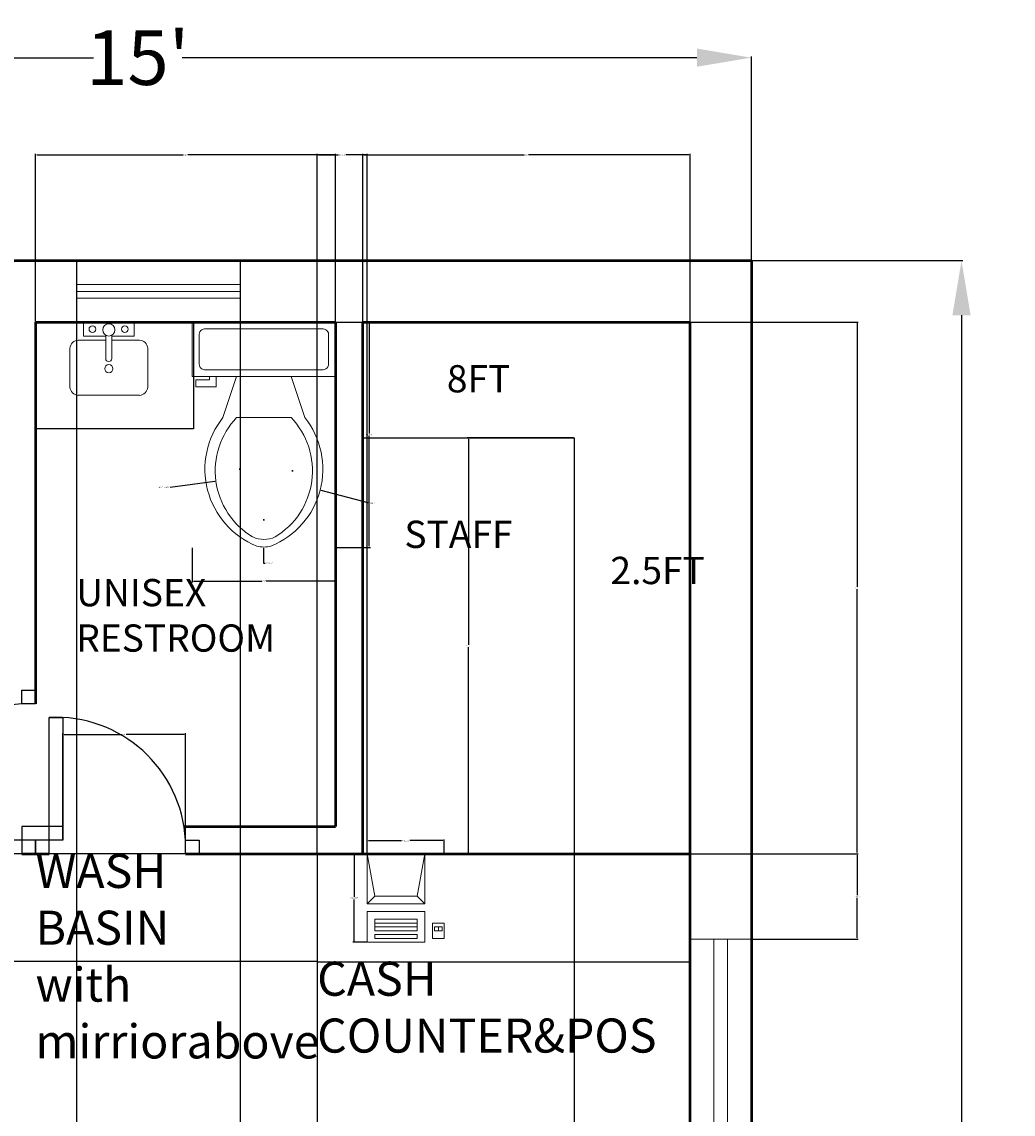
# Model space of a CAD drawing. Units: inches. Extents: x 226 to 1155, y 22 to 494.
# Tile 3 of 7: x 315 to 460, y 176 to 337. Entities that reach past the tile are written whole.
import ezdxf

# ---------------------------------------------------------------- set-up
doc = ezdxf.new("R2010")
doc.units = ezdxf.units.IN
doc.header["$MEASUREMENT"] = 0
for name, color, linetype, lineweight in [('A-ANNO-DIMS', 2, 'Continuous', 18), ('A-ANNO-TEXT', 7, 'Continuous', 18), ('A-AREA-IDEN', 7, 'Continuous', 25), ('A-DOOR', 3, 'Continuous', 25), ('A-EQPM', 8, 'Continuous', 18), ('A-FLOR-CASE', 9, 'Continuous', 25), ('A-FLOR-FIXT', 9, 'Continuous', 18), ('A-GLAZ', 4, 'Continuous', 18), ('A-WALL', 7, 'Continuous', 50)]:
    doc.layers.add(name, color=color, linetype=linetype, lineweight=lineweight)
doc.styles.get("Standard").update_dxf_attribs({"font": 'arial.ttf'})
doc.dimstyles.get("Standard").update_dxf_attribs({"dimtxt": 0.18, "dimasz": 0.18, "dimexe": 0.18, "dimexo": 0.0625, "dimgap": 0.09, "dimtad": 0, "dimtih": 1, "dimtoh": 1, "dimdec": 4, "dimzin": 0, "dimdsep": 46, "dimlunit": 4, "dimtxsty": 'Standard', "dimcen": 0.09, "dimadec": 0, "dimazin": 0, "dimtfac": 1, "dimtdec": 4, "dimtofl": 0, "dimtmove": 0, "dimatfit": 3, "dimfxl": 1, "dimtolj": 1, "dimtzin": 0, "dimarcsym": 0})

# ---------------------------------------------------------------- blocks, each defined once
blk = doc.blocks.new('Computer Terminal')
for p, q in [((-10, 11.5), (5, 11.5)), ((-8, 0.5), (-10, 11.5)), ((-10, -1.5), (-10, 11.5)), ((5, 11.5), (3, 0.5)), ((5, 11.5), (5, -1.5)), ((-10, -1.5), (-8, 0.5)), ((3, 0.5), (-8, 0.5)), ((3, 0.5), (5, -1.5)), ((5, -1.5), (-10, -1.5)), ((-10, -11.5), (-10, -3.5)), ((-10, -3.5), (5, -3.5)), ((-8, -5.5), (-8, -8.5)), ((3, -5.5), (-8, -5.5)), ((3, -8.5), (3, -5.5)), ((5, -3.5), (5, -11.5)), ((3, -6.5), (-8, -6.5)), ((-8, -7.5), (3, -7.5)), ((-8, -8.5), (3, -8.5)), ((10, -6.5), (7, -6.5)), ((7, -6.5), (7, -10.5)), ((9.5, -7.5), (7.5, -7.5)), ((7.5, -7.5), (7.5, -8.5)), ((7.5, -8.5), (9.5, -8.5)), ((8.5, -7.5), (8.5, -8.5)), ((9.5, -8.5), (9.5, -7.5)), ((10, -10.5), (10, -6.5)), ((-8, -9.5), (-8, -10.5)), ((3, -9.5), (-8, -9.5)), ((-8, -10.5), (3, -10.5)), ((3, -10.5), (3, -9.5)), ((7, -10.5), (10, -10.5)), ((5, -11.5), (-10, -11.5))]:
    blk.add_line(p, q)
blk = doc.blocks.new('Toilet - top')
for p, q in [((9.5, -6), (9.5, -2)), ((-8, -8.5), (-8, -8)), ((-7, -8), (-7, -9.5)), ((-4, -8), (-6, -14)), ((4, -8), (6, -14)), ((-10, -8.5), (-8, -8.5)), ((-10, -9.5), (-10, -8.5)), ((-7, -9.5), (-10, -9.5)), ((4, -14), (-4, -14))]:
    blk.add_line(p, q)
blk.add_lwpolyline([(10.5, -8), (10.5, 0), (-10.5, 0), (-10.5, -8)], close=True)
for points in [[(8.5, -1), (-8.5, -1)], [(-9.5, -2), (-9.5, -6)], [(-8.5, -7), (8.5, -7)]]:
    blk.add_lwpolyline(points)
for centre, radius, start, end in [((-8.62, -1.88), 0.884, 81.8699, 188.1301), ((8.62, -1.88), 0.884, 351.8699, 98.1301), ((-8.62, -6.12), 0.884, 171.8699, 278.1301), ((8.62, -6.12), 0.884, 261.8699, 8.1301), ((3.52, -21.58), 12.17, 141.4691, 247.9714), ((4.2, -21.82), 11.33, 136.3677, 238.9468), ((-3.52, -21.58), 12.17, 292.0284, 38.5307), ((-4.2, -21.82), 11.33, 301.053, 43.6321), ((0, -27.88), 4, 245.7318, 294.2682), ((0, -29), 4, 254.8605, 285.1395)]:
    blk.add_arc(centre, radius, start, end)
blk = doc.blocks.new('*D8')
at = {"layer": 'A-ANNO-DIMS', "color": 0, "lineweight": -2, "transparency": 16777216}
for p, q in [((421.77, 301.63), (452.71, 301.63)), ((452.53, 293.63), (452.53, 173.74)), ((452.53, 45.63), (452.53, 165.52)), ((421.77, 37.63), (452.71, 37.63))]:
    blk.add_line(p, q, dxfattribs=at)
at = {"layer": 'A-ANNO-DIMS', "color": 0, "transparency": 16777216}
for points in [[(451.2, 293.63), (453.86, 293.63), (452.53, 301.63)], [(451.2, 45.63), (453.86, 45.63), (452.53, 37.63)]]:
    blk.add_solid(points, dxfattribs=at)
at = {"layer": 'Defpoints', "color": 0, "transparency": 16777216}
for p in [(421.71, 301.63), (421.71, 37.63), (452.53, 37.63)]:
    blk.add_point(p, dxfattribs=at)
at = {"layer": 'A-ANNO-DIMS', "color": 0, "transparency": 16777216, "insert": (452.53, 169.63), "char_height": 8, "attachment_point": 5}
blk.add_mtext("\\A1;22'", dxfattribs=at)
blk = doc.blocks.new('*D9')
at = {"layer": 'A-ANNO-DIMS', "color": 0, "lineweight": -2, "transparency": 16777216}
for p, q in [((241.71, 301.69), (241.71, 331.58)), ((249.71, 331.4), (325.2, 331.4)), ((413.71, 331.4), (338.21, 331.4)), ((421.71, 301.69), (421.71, 331.58))]:
    blk.add_line(p, q, dxfattribs=at)
at = {"layer": 'A-ANNO-DIMS', "color": 0, "transparency": 16777216}
for points in [[(249.71, 332.74), (249.71, 330.07), (241.71, 331.4)], [(413.71, 332.74), (413.71, 330.07), (421.71, 331.4)]]:
    blk.add_solid(points, dxfattribs=at)
at = {"layer": 'Defpoints', "color": 0, "transparency": 16777216}
for p in [(421.71, 331.4), (241.71, 301.63), (421.71, 301.63)]:
    blk.add_point(p, dxfattribs=at)
at = {"layer": 'A-ANNO-DIMS', "color": 0, "transparency": 16777216, "insert": (331.71, 331.4), "char_height": 8, "attachment_point": 5}
blk.add_mtext("\\A1;15'", dxfattribs=at)
blk = doc.blocks.new('BASIN-WITH-FAUCET')
blk.add_line((6.15, 5.4), (6.15, 8.82))
for points in [[(5.25, 8.7), (2, 8.7), (2, 10.75), (5.8, 10.75)], [(5.8, 10.75), (9.4, 10.75), (9.4, 8.7), (6.15, 8.7)], [(1.2, 8.1), (5.25, 8.1)], [(6.15, 8.1), (10.2, 8.1)], [(0, 1.2), (0, 6.9)], [(11.4, 6.9), (11.4, 1.2)], [(10.2, 0), (1.2, 0)]]:
    blk.add_lwpolyline(points)
blk.add_lwpolyline([(6.15, 5.4, -1), (5.25, 5.4), (5.25, 8.82)], format="xyb")
for centre, radius in [((3.3, 9.7), 0.5), ((5.7, 9.6), 0.9), ((8.05, 9.7), 0.5), ((5.7, 3.9), 0.6)]:
    blk.add_circle(centre, radius)
for centre, start, end in [((1.28, 6.82), 93.3665, 176.6335), ((10.13, 6.82), 3.3665, 86.6335), ((1.28, 1.27), 183.3665, 266.6335), ((10.13, 1.27), 273.3665, 356.6335)]:
    blk.add_arc(centre, 1.28, start, end)
blk = doc.blocks.new('WIN-36')
for p, q in [((0, 5.5), (36, 5.5)), ((0, 3.5), (36, 3.5))]:
    blk.add_line(p, q)
blk.add_lwpolyline([(36, 9), (36, 0), (0, 0), (0, 9)], close=True)
blk = doc.blocks.new('*D46')
at = {"layer": 'A-ANNO-DIMS', "color": 0, "lineweight": -2, "transparency": 16777216}
for p, q in [((365.31, 214.63), (363.25, 214.63)), ((363.43, 214.45), (363.43, 208.33)), ((363.43, 201.84), (363.43, 207.96)), ((365.31, 201.66), (363.25, 201.66))]:
    blk.add_line(p, q, dxfattribs=at)
at = {"layer": 'A-ANNO-DIMS', "color": 0, "transparency": 16777216}
for points in [[(363.4, 214.45), (363.46, 214.45), (363.43, 214.63)], [(363.4, 201.84), (363.46, 201.84), (363.43, 201.66)]]:
    blk.add_solid(points, dxfattribs=at)
at = {"layer": 'Defpoints', "color": 0, "transparency": 16777216}
for p in [(363.43, 214.63), (365.38, 214.63), (365.38, 201.66)]:
    blk.add_point(p, dxfattribs=at)
at = {"layer": 'A-ANNO-DIMS', "color": 0, "transparency": 16777216, "insert": (363.43, 208.15), "char_height": 0.18, "attachment_point": 5}
blk.add_mtext('\\A1;POS 1\'-1"', dxfattribs=at)
blk = doc.blocks.new('*D47')
at = {"layer": 'A-ANNO-DIMS', "color": 0, "lineweight": -2, "transparency": 16777216}
for p, q in [((365.38, 214.69), (365.38, 216.76)), ((365.56, 216.58), (370.41, 216.58)), ((376.47, 216.58), (371.62, 216.58)), ((376.65, 214.69), (376.65, 216.76))]:
    blk.add_line(p, q, dxfattribs=at)
at = {"layer": 'A-ANNO-DIMS', "color": 0, "transparency": 16777216}
for points in [[(365.56, 216.61), (365.56, 216.55), (365.38, 216.58)], [(376.47, 216.61), (376.47, 216.55), (376.65, 216.58)]]:
    blk.add_solid(points, dxfattribs=at)
at = {"layer": 'Defpoints', "color": 0, "transparency": 16777216}
for p in [(376.65, 216.58), (365.38, 214.63), (376.65, 214.63)]:
    blk.add_point(p, dxfattribs=at)
at = {"layer": 'A-ANNO-DIMS', "color": 0, "transparency": 16777216, "insert": (371.01, 216.58), "char_height": 0.18, "attachment_point": 5}
blk.add_mtext('\\A1;0\'-11 1/2"', dxfattribs=at)
blk = doc.blocks.new('*D54')
at = {"layer": 'A-ANNO-DIMS', "color": 0, "lineweight": -2, "transparency": 16777216}
for p, q in [((360.77, 292.63), (365.84, 292.63)), ((365.66, 292.45), (365.66, 276.29)), ((365.66, 259.76), (365.66, 275.92)), ((360.77, 259.58), (365.84, 259.58))]:
    blk.add_line(p, q, dxfattribs=at)
at = {"layer": 'A-ANNO-DIMS', "color": 0, "transparency": 16777216}
for points in [[(365.63, 292.45), (365.69, 292.45), (365.66, 292.63)], [(365.63, 259.76), (365.69, 259.76), (365.66, 259.58)]]:
    blk.add_solid(points, dxfattribs=at)
at = {"layer": 'Defpoints', "color": 0, "transparency": 16777216}
for p in [(360.71, 292.63), (365.66, 292.63), (360.71, 259.58)]:
    blk.add_point(p, dxfattribs=at)
at = {"layer": 'A-ANNO-DIMS', "color": 0, "transparency": 16777216, "insert": (365.66, 276.11), "char_height": 0.18, "attachment_point": 5}
blk.add_mtext('\\A1;WC 2\'-9"', dxfattribs=at)
blk = doc.blocks.new('*D55')
at = {"layer": 'A-ANNO-DIMS', "color": 0, "lineweight": -2, "transparency": 16777216}
for p, q in [((339.71, 259.52), (339.71, 254.45)), ((360.71, 259.52), (360.71, 254.45)), ((339.89, 254.63), (349.89, 254.63)), ((360.53, 254.63), (350.53, 254.63))]:
    blk.add_line(p, q, dxfattribs=at)
at = {"layer": 'A-ANNO-DIMS', "color": 0, "transparency": 16777216}
for points in [[(339.89, 254.66), (339.89, 254.6), (339.71, 254.63)], [(360.53, 254.66), (360.53, 254.6), (360.71, 254.63)]]:
    blk.add_solid(points, dxfattribs=at)
at = {"layer": 'Defpoints', "color": 0, "transparency": 16777216}
for p in [(339.71, 259.58), (360.71, 259.58), (360.71, 254.63)]:
    blk.add_point(p, dxfattribs=at)
at = {"layer": 'A-ANNO-DIMS', "color": 0, "transparency": 16777216, "insert": (350.21, 254.63), "char_height": 0.18, "attachment_point": 5}
blk.add_mtext('\\A1;1\'-9"', dxfattribs=at)
blk = doc.blocks.new('*D57')
at = {"layer": 'A-ANNO-DIMS', "color": 0, "lineweight": -2, "transparency": 16777216}
for p, q in [((316.71, 292.69), (316.71, 317.31)), ((360.71, 292.69), (360.71, 317.31)), ((316.89, 317.13), (338.38, 317.13)), ((360.53, 317.13), (339.04, 317.13))]:
    blk.add_line(p, q, dxfattribs=at)
at = {"layer": 'A-ANNO-DIMS', "color": 0, "transparency": 16777216}
for points in [[(316.89, 317.16), (316.89, 317.1), (316.71, 317.13)], [(360.53, 317.16), (360.53, 317.1), (360.71, 317.13)]]:
    blk.add_solid(points, dxfattribs=at)
at = {"layer": 'Defpoints', "color": 0, "transparency": 16777216}
for p in [(360.71, 317.13), (316.71, 292.63), (360.71, 292.63)]:
    blk.add_point(p, dxfattribs=at)
at = {"layer": 'A-ANNO-DIMS', "color": 0, "transparency": 16777216, "insert": (338.71, 317.13), "char_height": 0.18, "attachment_point": 5}
blk.add_mtext('\\A1;3\'-8"', dxfattribs=at)
blk = doc.blocks.new('*D58')
at = {"layer": 'A-ANNO-DIMS', "color": 0, "lineweight": -2, "transparency": 16777216}
for p, q in [((364.71, 292.69), (364.71, 317.31)), ((412.71, 292.69), (412.71, 317.31)), ((364.89, 317.13), (388.37, 317.13)), ((412.53, 317.13), (389.04, 317.13))]:
    blk.add_line(p, q, dxfattribs=at)
at = {"layer": 'A-ANNO-DIMS', "color": 0, "transparency": 16777216}
for points in [[(364.89, 317.16), (364.89, 317.1), (364.71, 317.13)], [(412.53, 317.16), (412.53, 317.1), (412.71, 317.13)]]:
    blk.add_solid(points, dxfattribs=at)
at = {"layer": 'Defpoints', "color": 0, "transparency": 16777216}
for p in [(412.71, 317.13), (364.71, 292.63), (412.71, 292.63)]:
    blk.add_point(p, dxfattribs=at)
at = {"layer": 'A-ANNO-DIMS', "color": 0, "transparency": 16777216, "insert": (388.71, 317.13), "char_height": 0.18, "attachment_point": 5}
blk.add_mtext('\\A1;4\'-0"', dxfattribs=at)
blk = doc.blocks.new('*D60')
at = {"layer": 'A-ANNO-DIMS', "color": 0, "lineweight": -2, "transparency": 16777216}
for p, q in [((412.77, 292.63), (437.39, 292.63)), ((437.21, 292.45), (437.21, 253.81)), ((437.21, 214.81), (437.21, 253.45)), ((412.77, 214.63), (437.39, 214.63))]:
    blk.add_line(p, q, dxfattribs=at)
at = {"layer": 'A-ANNO-DIMS', "color": 0, "transparency": 16777216}
for points in [[(437.18, 292.45), (437.24, 292.45), (437.21, 292.63)], [(437.18, 214.81), (437.24, 214.81), (437.21, 214.63)]]:
    blk.add_solid(points, dxfattribs=at)
at = {"layer": 'Defpoints', "color": 0, "transparency": 16777216}
for p in [(412.71, 292.63), (437.21, 292.63), (412.71, 214.63)]:
    blk.add_point(p, dxfattribs=at)
at = {"layer": 'A-ANNO-DIMS', "color": 0, "transparency": 16777216, "insert": (437.21, 253.63), "char_height": 0.18, "attachment_point": 5}
blk.add_mtext('\\A1;6\'-6"', dxfattribs=at)
blk = doc.blocks.new('*D66')
at = {"layer": 'A-ANNO-DIMS', "color": 0, "lineweight": -2, "transparency": 16777216}
for p, q in [((412.77, 214.63), (437.39, 214.63)), ((437.21, 214.45), (437.21, 208.56)), ((437.21, 202.29), (437.21, 208.19)), ((421.77, 202.11), (437.39, 202.11))]:
    blk.add_line(p, q, dxfattribs=at)
at = {"layer": 'A-ANNO-DIMS', "color": 0, "transparency": 16777216}
for points in [[(437.18, 214.45), (437.24, 214.45), (437.21, 214.63)], [(437.18, 202.29), (437.24, 202.29), (437.21, 202.11)]]:
    blk.add_solid(points, dxfattribs=at)
at = {"layer": 'Defpoints', "color": 0, "transparency": 16777216}
for p in [(412.71, 214.63), (437.21, 214.63), (421.71, 202.11)]:
    blk.add_point(p, dxfattribs=at)
at = {"layer": 'A-ANNO-DIMS', "color": 0, "transparency": 16777216, "insert": (437.21, 208.37), "char_height": 0.18, "attachment_point": 5}
blk.add_mtext('\\A1;1\'-0 1/2"', dxfattribs=at)
blk = doc.blocks.new('*D71')
at = {"layer": 'A-ANNO-DIMS', "color": 0, "lineweight": -2, "transparency": 16777216}
for p, q in [((241.71, 301.57), (241.71, 21.95)), ((322.71, 301.57), (322.71, 21.95)), ((241.89, 22.13), (281.88, 22.13)), ((322.53, 22.13), (282.54, 22.13))]:
    blk.add_line(p, q, dxfattribs=at)
at = {"layer": 'A-ANNO-DIMS', "color": 0, "transparency": 16777216}
for points in [[(241.89, 22.16), (241.89, 22.1), (241.71, 22.13)], [(322.53, 22.16), (322.53, 22.1), (322.71, 22.13)]]:
    blk.add_solid(points, dxfattribs=at)
at = {"layer": 'Defpoints', "color": 0, "transparency": 16777216}
for p in [(241.71, 301.63), (322.71, 301.63), (322.71, 22.13)]:
    blk.add_point(p, dxfattribs=at)
at = {"layer": 'A-ANNO-DIMS', "color": 0, "transparency": 16777216, "insert": (282.21, 22.13), "char_height": 0.18, "attachment_point": 5}
blk.add_mtext('\\A1;6\'-9"', dxfattribs=at)
blk = doc.blocks.new('*D72')
at = {"layer": 'A-ANNO-DIMS', "color": 0, "lineweight": -2, "transparency": 16777216}
for p, q in [((322.71, 301.57), (322.71, 21.95)), ((346.71, 301.57), (346.71, 21.95)), ((322.89, 22.13), (334.38, 22.13)), ((346.53, 22.13), (335.04, 22.13))]:
    blk.add_line(p, q, dxfattribs=at)
at = {"layer": 'A-ANNO-DIMS', "color": 0, "transparency": 16777216}
for points in [[(322.89, 22.16), (322.89, 22.1), (322.71, 22.13)], [(346.53, 22.16), (346.53, 22.1), (346.71, 22.13)]]:
    blk.add_solid(points, dxfattribs=at)
at = {"layer": 'Defpoints', "color": 0, "transparency": 16777216}
for p in [(322.71, 301.63), (346.71, 301.63), (346.71, 22.13)]:
    blk.add_point(p, dxfattribs=at)
at = {"layer": 'A-ANNO-DIMS', "color": 0, "transparency": 16777216, "insert": (334.71, 22.13), "char_height": 0.18, "attachment_point": 5}
blk.add_mtext('\\A1;2\'-0"', dxfattribs=at)
blk = doc.blocks.new('*D81')
at = {"layer": 'A-ANNO-DIMS', "color": 0, "lineweight": -2, "transparency": 16777216}
for p, q in [((358.02, 198.75), (358.02, 21.95)), ((412.71, 198.75), (412.71, 21.95)), ((358.2, 22.13), (384.82, 22.13)), ((412.53, 22.13), (385.91, 22.13))]:
    blk.add_line(p, q, dxfattribs=at)
at = {"layer": 'A-ANNO-DIMS', "color": 0, "transparency": 16777216}
for points in [[(358.2, 22.16), (358.2, 22.1), (358.02, 22.13)], [(412.53, 22.16), (412.53, 22.1), (412.71, 22.13)]]:
    blk.add_solid(points, dxfattribs=at)
at = {"layer": 'Defpoints', "color": 0, "transparency": 16777216}
for p in [(358.02, 198.82), (412.71, 198.82), (412.71, 22.13)]:
    blk.add_point(p, dxfattribs=at)
at = {"layer": 'A-ANNO-DIMS', "color": 0, "transparency": 16777216, "insert": (385.36, 22.13), "char_height": 0.18, "attachment_point": 5}
blk.add_mtext('\\A1;4\'-6 1/2"', dxfattribs=at)
blk = doc.blocks.new('*D82')
at = {"layer": 'A-ANNO-DIMS', "color": 0, "lineweight": -2, "transparency": 16777216}
for p, q in [((357.96, 214.63), (226.03, 214.63)), ((226.21, 214.45), (226.21, 206.9)), ((226.21, 199), (226.21, 206.54)), ((357.96, 198.82), (226.03, 198.82))]:
    blk.add_line(p, q, dxfattribs=at)
at = {"layer": 'A-ANNO-DIMS', "color": 0, "transparency": 16777216}
for points in [[(226.18, 214.45), (226.24, 214.45), (226.21, 214.63)], [(226.18, 199), (226.24, 199), (226.21, 198.82)]]:
    blk.add_solid(points, dxfattribs=at)
at = {"layer": 'Defpoints', "color": 0, "transparency": 16777216}
for p in [(226.21, 214.63), (358.02, 214.63), (358.02, 198.82)]:
    blk.add_point(p, dxfattribs=at)
at = {"layer": 'A-ANNO-DIMS', "color": 0, "transparency": 16777216, "insert": (226.21, 206.72), "char_height": 0.18, "attachment_point": 5}
blk.add_mtext('\\A1;1\'-4"', dxfattribs=at)
blk = doc.blocks.new('*D83')
at = {"layer": 'A-ANNO-DIMS', "color": 0, "lineweight": -2, "transparency": 16777216}
for p, q in [((358.02, 214.69), (358.02, 317.31)), ((365.38, 214.69), (365.38, 317.31)), ((358.2, 317.13), (361.16, 317.13)), ((365.2, 317.13), (362.24, 317.13))]:
    blk.add_line(p, q, dxfattribs=at)
at = {"layer": 'A-ANNO-DIMS', "color": 0, "transparency": 16777216}
for points in [[(358.2, 317.16), (358.2, 317.1), (358.02, 317.13)], [(365.2, 317.16), (365.2, 317.1), (365.38, 317.13)]]:
    blk.add_solid(points, dxfattribs=at)
at = {"layer": 'Defpoints', "color": 0, "transparency": 16777216}
for p in [(365.38, 317.13), (358.02, 214.63), (365.38, 214.63)]:
    blk.add_point(p, dxfattribs=at)
at = {"layer": 'A-ANNO-DIMS', "color": 0, "transparency": 16777216, "insert": (361.7, 317.13), "char_height": 0.18, "attachment_point": 5}
blk.add_mtext('\\A1;0\'-7 1/2"', dxfattribs=at)
blk = doc.blocks.new('*D84')
at = {"layer": 'A-ANNO-DIMS', "color": 0, "lineweight": -2, "transparency": 16777216}
for p, q in [((412.71, 292.57), (412.71, 21.95)), ((395.71, 275.57), (395.71, 21.95)), ((395.89, 22.13), (403.89, 22.13)), ((412.53, 22.13), (404.53, 22.13))]:
    blk.add_line(p, q, dxfattribs=at)
at = {"layer": 'A-ANNO-DIMS', "color": 0, "transparency": 16777216}
for points in [[(395.89, 22.16), (395.89, 22.1), (395.71, 22.13)], [(412.53, 22.16), (412.53, 22.1), (412.71, 22.13)]]:
    blk.add_solid(points, dxfattribs=at)
at = {"layer": 'Defpoints', "color": 0, "transparency": 16777216}
for p in [(412.71, 292.63), (395.71, 275.63), (412.71, 22.13)]:
    blk.add_point(p, dxfattribs=at)
at = {"layer": 'A-ANNO-DIMS', "color": 0, "transparency": 16777216, "insert": (404.21, 22.13), "char_height": 0.18, "attachment_point": 5}
blk.add_mtext('\\A1;1\'-5"', dxfattribs=at)
blk = doc.blocks.new('*D85')
at = {"layer": 'A-ANNO-DIMS', "color": 0, "lineweight": -2, "transparency": 16777216}
for p, q in [((395.64, 275.63), (380.03, 275.63)), ((380.21, 275.45), (380.21, 245.31)), ((380.21, 214.81), (380.21, 244.95)), ((395.64, 214.63), (380.03, 214.63))]:
    blk.add_line(p, q, dxfattribs=at)
at = {"layer": 'A-ANNO-DIMS', "color": 0, "transparency": 16777216}
for points in [[(380.18, 275.45), (380.24, 275.45), (380.21, 275.63)], [(380.18, 214.81), (380.24, 214.81), (380.21, 214.63)]]:
    blk.add_solid(points, dxfattribs=at)
at = {"layer": 'Defpoints', "color": 0, "transparency": 16777216}
for p in [(380.21, 275.63), (395.71, 275.63), (395.71, 214.63)]:
    blk.add_point(p, dxfattribs=at)
at = {"layer": 'A-ANNO-DIMS', "color": 0, "transparency": 16777216, "insert": (380.21, 245.13), "char_height": 0.18, "attachment_point": 5}
blk.add_mtext('\\A1;5\'-1"', dxfattribs=at)
blk = doc.blocks.new('*D90')
at = {"layer": 'A-ANNO-DIMS', "color": 0, "lineweight": -2, "transparency": 16777216}
for p, q in [((320.71, 216.69), (320.71, 232.31)), ((338.71, 216.69), (338.71, 232.31)), ((320.89, 232.13), (329.39, 232.13)), ((338.53, 232.13), (330.03, 232.13))]:
    blk.add_line(p, q, dxfattribs=at)
at = {"layer": 'A-ANNO-DIMS', "color": 0, "transparency": 16777216}
for points in [[(320.89, 232.16), (320.89, 232.1), (320.71, 232.13)], [(338.53, 232.16), (338.53, 232.1), (338.71, 232.13)]]:
    blk.add_solid(points, dxfattribs=at)
at = {"layer": 'Defpoints', "color": 0, "transparency": 16777216}
for p in [(338.71, 232.13), (320.71, 216.63), (338.71, 216.63)]:
    blk.add_point(p, dxfattribs=at)
at = {"layer": 'A-ANNO-DIMS', "color": 0, "transparency": 16777216, "insert": (329.71, 232.13), "char_height": 0.18, "attachment_point": 5}
blk.add_mtext('\\A1;1\'-6"', dxfattribs=at)
blk = doc.blocks.new('*D120')
at = {"layer": 'A-ANNO-DIMS', "color": 0, "lineweight": -2, "transparency": 16777216}
for p, q in [((346.6, 271.05), (346.78, 271.05)), ((346.69, 270.96), (346.69, 271.14)), ((365.52, 266.1), (358.63, 267.91))]:
    blk.add_line(p, q, dxfattribs=at)
at = {"layer": 'A-ANNO-DIMS', "color": 0, "transparency": 16777216}
blk.add_solid([(358.64, 267.94), (358.62, 267.88), (358.46, 267.96)], dxfattribs=at)
at = {"layer": 'Defpoints', "color": 0, "transparency": 16777216}
for p in [(346.69, 271.05), (358.46, 267.96)]:
    blk.add_point(p, dxfattribs=at)
at = {"layer": 'A-ANNO-DIMS', "color": 0, "transparency": 16777216, "insert": (366.13, 266.1), "char_height": 0.18, "attachment_point": 5}
blk.add_mtext('\\A1;2X R1\'-0"', dxfattribs=at)
blk = doc.blocks.new('*D121')
at = {"layer": 'A-ANNO-DIMS', "color": 0, "lineweight": -2, "transparency": 16777216}
for p, q in [((354.32, 270.81), (354.5, 270.81)), ((354.41, 270.72), (354.41, 270.9)), ((336.44, 268.4), (343, 269.28))]:
    blk.add_line(p, q, dxfattribs=at)
at = {"layer": 'A-ANNO-DIMS', "color": 0, "transparency": 16777216}
blk.add_solid([(343, 269.31), (343, 269.25), (343.18, 269.3)], dxfattribs=at)
at = {"layer": 'Defpoints', "color": 0, "transparency": 16777216}
for p in [(354.41, 270.81), (343.18, 269.3)]:
    blk.add_point(p, dxfattribs=at)
at = {"layer": 'A-ANNO-DIMS', "color": 0, "transparency": 16777216, "insert": (335.55, 268.4), "char_height": 0.18, "attachment_point": 5}
blk.add_mtext('\\A1;2X R0\'-11 1/2"', dxfattribs=at)
blk = doc.blocks.new('*D122')
at = {"layer": 'A-ANNO-DIMS', "color": 0, "lineweight": -2, "transparency": 16777216}
for p, q in [((350.12, 263.63), (350.3, 263.63)), ((350.21, 263.54), (350.21, 263.72)), ((350.21, 257.23), (350.21, 259.45)), ((350.39, 257.23), (350.21, 257.23))]:
    blk.add_line(p, q, dxfattribs=at)
at = {"layer": 'A-ANNO-DIMS', "color": 0, "transparency": 16777216}
blk.add_solid([(350.24, 259.45), (350.18, 259.45), (350.21, 259.63)], dxfattribs=at)
at = {"layer": 'Defpoints', "color": 0, "transparency": 16777216}
for p in [(350.21, 263.63), (350.21, 259.63)]:
    blk.add_point(p, dxfattribs=at)
at = {"layer": 'A-ANNO-DIMS', "color": 0, "transparency": 16777216, "insert": (351, 257.23), "char_height": 0.18, "attachment_point": 5}
blk.add_mtext('\\A1;2X R0\'-4"', dxfattribs=at)

msp = doc.modelspace()

# ---------------------------------------------------------------- linework, layer by layer
at = {"layer": 'A-DOOR'}
for p, q in [((316.70585, 236.62988), (316.70585, 238.62988)), ((316.70585, 214.62988), (316.70585, 216.62988)), ((316.70585, 214.62988), (318.70585, 214.62988)), ((338.70585, 214.62988), (340.70585, 214.62988))]:
    msp.add_line(p, q, dxfattribs=at)
for points in [[(316.70585, 238.62988), (316.70585, 236.62988), (314.70585, 236.62988), (314.70585, 238.62988)], [(316.70585, 214.62988), (316.70585, 216.62988), (314.70585, 216.62988), (314.70585, 214.62988)], [(316.70585, 214.62988), (318.70585, 214.62988), (318.70585, 216.62988), (316.70585, 216.62988)], [(340.70585, 214.62988), (338.70585, 214.62988), (338.70585, 216.62988), (340.70585, 216.62988)]]:
    msp.add_lwpolyline(points, close=True, dxfattribs=at)
for points in [[(314.70585, 236.62988, 0.414213562), (296.70585, 216.62988), (296.70585, 218.62988)], [(338.70585, 216.62988, 0.414213562), (318.70585, 234.62988), (320.70585, 234.62988), (320.70585, 216.62988), (318.70585, 216.62988), (318.70585, 234.62988)]]:
    msp.add_lwpolyline(points, format="xyb", dxfattribs=at)
msp.add_lwpolyline([(320.70585, 218.62988), (314.70585, 218.62988), (314.70585, 216.62988), (296.70585, 216.62988)], dxfattribs=at)
at = {"layer": 'A-EQPM'}
msp.add_line((365.37517, 214.62988), (373.83336, 214.62988), dxfattribs=at)
at = {"layer": 'A-FLOR-CASE'}
msp.add_lwpolyline([(316.70585, 292.62988), (339.86098, 292.62988), (339.86098, 276.95966), (316.70585, 276.95966)], close=True, dxfattribs=at)
for points in [[(364.70585, 275.62988), (395.70585, 275.62988), (395.70585, 214.62988)], [(358.02219, 214.62988), (358.02219, 198.81719), (412.70585, 198.81719)]]:
    msp.add_lwpolyline(points, dxfattribs=at)
at = {"layer": 'A-GLAZ'}
for p, q in [((322.7094, 298.12988), (346.7094, 298.12988)), ((322.7094, 297.12988), (346.7094, 297.12988)), ((322.7094, 296.12988), (346.7094, 296.12988))]:
    msp.add_line(p, q, dxfattribs=at)
msp.add_lwpolyline([(346.7094, 301.62988), (346.7094, 292.62988), (322.7094, 292.62988), (322.7094, 301.62988)], close=True, dxfattribs=at)
at = {"layer": 'A-WALL'}
for p, q in [((316.70585, 292.62988), (316.70585, 236.62988)), ((316.70585, 292.62988), (360.70585, 292.62988)), ((360.70585, 292.62988), (360.70585, 218.62988)), ((338.49414, 218.62988), (360.70585, 218.62988)), ((314.70585, 214.62988), (318.70585, 214.62988)), ((338.70585, 214.62988), (412.70585, 214.62988))]:
    msp.add_line(p, q, dxfattribs=at)
for points in [[(307.38052, 37.62988), (241.70585, 37.62988), (241.70585, 301.62988), (421.70585, 301.62988), (421.70585, 37.62988), (351.38052, 37.62988)], [(364.70585, 214.62988), (364.70585, 292.62988), (412.70585, 292.62988), (412.70585, 46.62988), (349.38052, 46.62988)]]:
    msp.add_lwpolyline(points, dxfattribs=at)

# ---------------------------------------------------------------- block references
at = {"layer": 'A-EQPM', "xscale": 0.56387934998791, "yscale": 0.56387934998791, "zscale": 0.56387934998791}
msp.add_blockref('Computer Terminal', (371.01397, 208.14526), dxfattribs=at)
at = {"layer": 'A-FLOR-FIXT'}
for name, p in [('BASIN-WITH-FAUCET', (321.761, 281.88)), ('Toilet - top', (350.20585, 292.62988))]:
    msp.add_blockref(name, p, dxfattribs=at)
at = {"layer": 'A-GLAZ', "rotation": 270}
msp.add_blockref('WIN-36', (412.70597, 202.11457), dxfattribs=at)

# ---------------------------------------------------------------- texts
at = {"layer": 'A-ANNO-TEXT', "attachment_point": 1}
for s, width, insert, char_height in [('8FT', 14.5329901, (377.0411, 286.3119), 4), ('2.5FT', 7.61252, (401.03207, 258.19169), 4), ('WASH BASIN\\Pwith mirriorabove', 32.3909522, (316.70585, 214.62988), 5), ('CASH COUNTER&POS', 54.6836594, (358.02219, 198.81719), 5)]:
    msp.add_mtext_dynamic_manual_height_columns(s, width=width, gutter_width=1, heights=[0], dxfattribs=dict(at, insert=insert, char_height=char_height))
at = {"layer": 'A-AREA-IDEN', "char_height": 4, "attachment_point": 1}
for s, width, insert in [('STAFF ', 21.2227815, (370.81267, 263.49304)), ('UNISEX\\PRESTROOM', 38.0282515, (322.67759, 254.94662))]:
    msp.add_mtext_dynamic_manual_height_columns(s, width=width, gutter_width=1, heights=[0], dxfattribs=dict(at, insert=insert))

# ---------------------------------------------------------------- dimensions: what is measured, and where the dimension line sits
at = {"layer": 'A-ANNO-DIMS'}
for base, p1, p2, override, picture, middle in [((421.70585, 331.40497), (241.70585, 301.62988), (421.70585, 301.62988), {"dimtxt": 8, "dimasz": 8, "dimclrd": 0, "dimclre": 0, "dimclrt": 0}, '*D9', (331.70585, 331.40497)), ((360.70585, 317.12988), (316.70585, 292.62988), (360.70585, 292.62988), {"dimdec": 1, "dimlfac": 1, "dimrnd": 0, "dimzin": 1, "dimdsep": 46, "dimlunit": 4, "dimfrac": 2}, '*D57', (338.70585, 317.12988)), ((365.37517, 317.12988), (358.02219, 214.62988), (365.37517, 214.62988), {"dimdec": 1, "dimlfac": 1, "dimrnd": 0, "dimzin": 1, "dimdsep": 46, "dimlunit": 4, "dimfrac": 2}, '*D83', (361.69868, 317.12988)), ((412.70584, 317.12988), (364.70585, 292.62988), (412.70584, 292.62988), {"dimdec": 1, "dimlfac": 1, "dimrnd": 0, "dimzin": 1, "dimdsep": 46, "dimlunit": 4, "dimfrac": 2}, '*D58', (388.70585, 317.12988)), ((322.7094, 22.12988), (241.70585, 301.62988), (322.7094, 301.62988), {"dimdec": 1, "dimlfac": 1, "dimrnd": 0, "dimzin": 1, "dimdsep": 46, "dimlunit": 4, "dimfrac": 2}, '*D71', (282.20762, 22.12988)), ((346.7094, 22.12988), (322.7094, 301.62988), (346.7094, 301.62988), {"dimdec": 1, "dimlfac": 1, "dimrnd": 0, "dimzin": 1, "dimdsep": 46, "dimlunit": 4, "dimfrac": 2}, '*D72', (334.7094, 22.12988)), ((412.70584, 22.12988), (395.70585, 275.62988), (412.70584, 292.62988), {"dimdec": 1, "dimlfac": 1, "dimrnd": 0, "dimzin": 1, "dimdsep": 46, "dimlunit": 4, "dimfrac": 2}, '*D84', (404.20584, 22.12988)), ((360.70585, 254.6267), (339.70585, 259.58363), (360.70585, 259.58363), {"dimdec": 1, "dimlfac": 1, "dimrnd": 0, "dimzin": 1, "dimdsep": 46, "dimlunit": 4, "dimfrac": 2}, '*D55', (350.20585, 254.6267)), ((338.70585, 232.12988), (320.70585, 216.62988), (338.70585, 216.62988), {"dimdec": 1, "dimlfac": 1, "dimrnd": 0, "dimzin": 1, "dimdsep": 46, "dimlunit": 4, "dimfrac": 2}, '*D90', (329.70585, 232.12988)), ((376.65276, 216.57526), (365.37517, 214.62988), (376.65276, 214.62988), {"dimdec": 1, "dimlfac": 1, "dimrnd": 0, "dimzin": 1, "dimdsep": 46, "dimlunit": 4, "dimfrac": 2}, '*D47', (371.01397, 216.57526)), ((412.70584, 22.12988), (358.02219, 198.81719), (412.70584, 198.81719), {"dimdec": 1, "dimlfac": 1, "dimrnd": 0, "dimzin": 1, "dimdsep": 46, "dimlunit": 4, "dimfrac": 2}, '*D81', (385.36402, 22.12988))]:
    dim = msp.add_linear_dim(base=base, p1=p1, p2=p2, dimstyle='Standard', override=override, dxfattribs=at)
    dim.commit()
    dim.dimension.update_dxf_attribs({"geometry": picture, "text_midpoint": middle})
for base, p1, p2, override, picture, middle in [((452.53152, 37.62988), (421.70585, 301.62988), (421.70585, 37.62988), {"dimtxt": 8, "dimasz": 8, "dimclrd": 0, "dimclre": 0, "dimclrt": 0}, '*D8', (452.53152, 169.62988)), ((437.20585, 292.62988), (412.70584, 214.62988), (412.70584, 292.62988), {"dimdec": 1, "dimlfac": 1, "dimrnd": 0, "dimzin": 1, "dimdsep": 46, "dimlunit": 4, "dimfrac": 2}, '*D60', (437.20585, 253.62988)), ((380.20585, 275.62988), (395.70585, 214.62988), (395.70585, 275.62988), {"dimdec": 1, "dimlfac": 1, "dimrnd": 0, "dimzin": 1, "dimdsep": 46, "dimlunit": 4, "dimfrac": 2}, '*D85', (380.20585, 245.12988)), ((226.20585, 214.62988), (358.02219, 198.81719), (358.02219, 214.62988), {"dimdec": 1, "dimlfac": 1, "dimrnd": 0, "dimzin": 1, "dimdsep": 46, "dimlunit": 4, "dimfrac": 2}, '*D82', (226.20585, 206.72354)), ((437.20585, 214.62988), (421.70585, 202.11428), (412.70584, 214.62988), {"dimdec": 1, "dimlfac": 1, "dimrnd": 0, "dimzin": 1, "dimdsep": 46, "dimlunit": 4, "dimfrac": 2}, '*D66', (437.20585, 208.37208))]:
    dim = msp.add_linear_dim(base=base, p1=p1, p2=p2, angle=90, dimstyle='Standard', override=override, dxfattribs=at)
    dim.commit()
    dim.dimension.update_dxf_attribs({"geometry": picture, "text_midpoint": middle})
for base, p1, p2, text, picture, middle in [((365.66278, 292.62988), (360.70585, 259.58363), (360.70585, 292.62988), 'WC <>', '*D54', (365.66278, 276.10676)), ((363.42979, 214.62988), (365.37517, 201.66064), (365.37517, 214.62988), 'POS <>', '*D46', (363.42979, 208.14526))]:
    dim = msp.add_linear_dim(base=base, p1=p1, p2=p2, angle=90, text=text, dimstyle='Standard', override={"dimdec": 1, "dimlfac": 1, "dimrnd": 0, "dimzin": 1, "dimdsep": 46, "dimlunit": 4, "dimfrac": 2}, dxfattribs=at)
    dim.commit()
    dim.dimension.update_dxf_attribs({"geometry": picture, "text_midpoint": middle})
for center, mpoint, picture, middle in [((354.4058, 270.81247), (343.17764, 269.30295), '*D121', (336.44074, 268.39724)), ((346.68635, 271.04941), (358.45591, 267.95702), '*D120', (365.51764, 266.1016)), ((350.20587, 263.62991), (350.206, 259.62991), '*D122', (350.99637, 257.22991))]:
    dim = msp.add_radius_dim(center=center, mpoint=mpoint, text='2X <>', dimstyle='Standard', override={"dimdec": 1, "dimlfac": 1, "dimrnd": 0, "dimzin": 1, "dimdsep": 46, "dimlunit": 4, "dimfrac": 2}, dxfattribs=at)
    dim.commit()
    dim.dimension.update_dxf_attribs({"geometry": picture, "text_midpoint": middle, "dimtype": 164})

doc.saveas('drawing.dxf')
